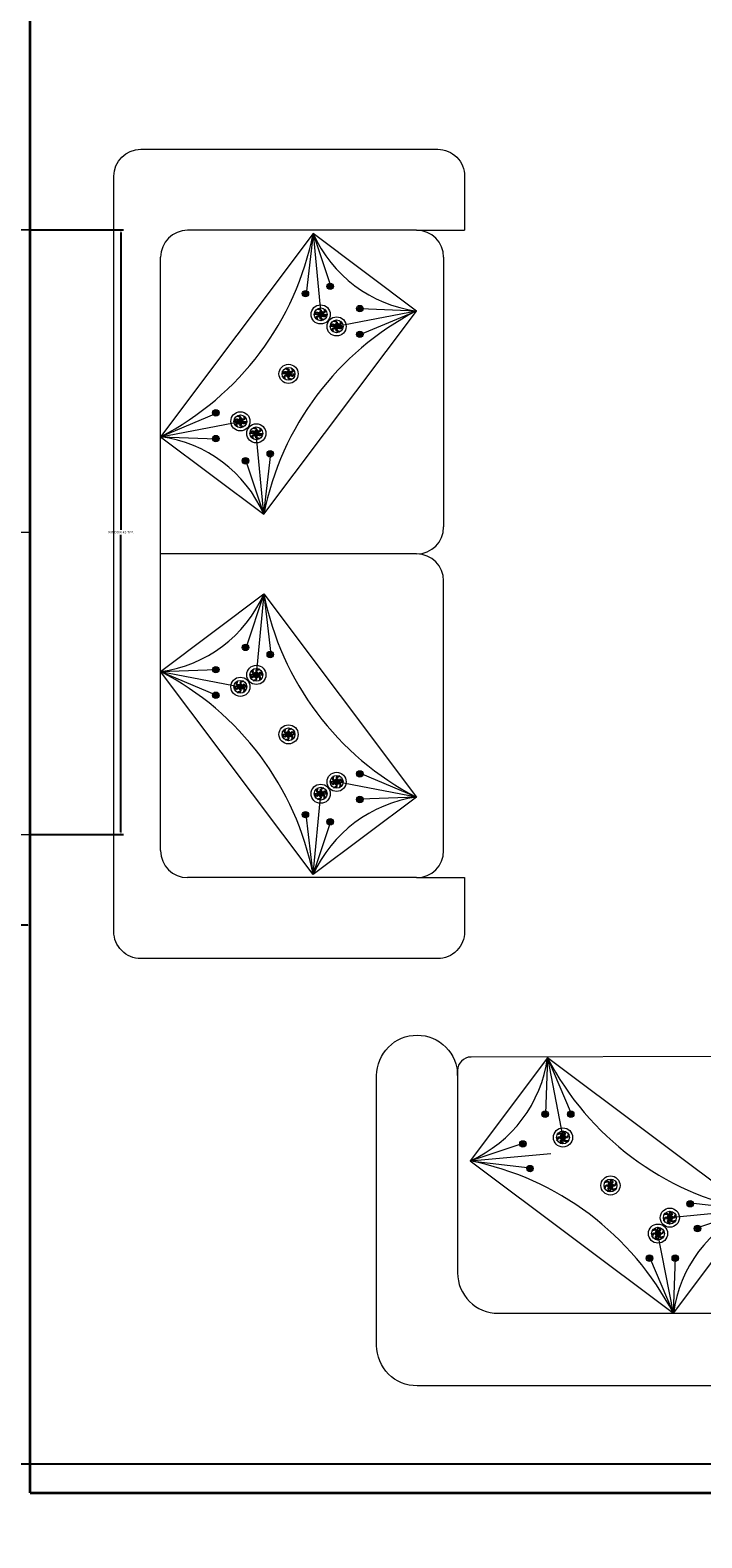
# Model space of a CAD drawing. Units: inches. Extents: x -61 to 1599, y -1316 to 257.
# Tile 193 of 204: x 1098 to 1147, y -173 to -61. Entities that reach past the tile are written whole.
import ezdxf

# ---------------------------------------------------------------- set-up
doc = ezdxf.new("R2010")
doc.units = ezdxf.units.IN
doc.header["$MEASUREMENT"] = 0
for name, color, linetype, lineweight in [('A-ANNO-DIMS', 2, 'Continuous', 18), ('FURNITURE', 83, 'Continuous', 18), ('WALLS', 4, 'Continuous', 35), ('WINDOWS', 220, 'Continuous', 18)]:
    doc.layers.add(name, color=color, linetype=linetype, lineweight=lineweight)
doc.layers.add('FUR', color=83, linetype='Continuous')
doc.styles.get("Standard").update_dxf_attribs({"font": 'arial.ttf'})
doc.dimstyles.get("Standard").update_dxf_attribs({"dimtxt": 0.18, "dimasz": 0.18, "dimexe": 0.18, "dimexo": 0.0625, "dimgap": 0.09, "dimtad": 0, "dimtih": 1, "dimtoh": 1, "dimdec": 0, "dimzin": 0, "dimdsep": 46, "dimlunit": 3, "dimtxsty": 'Standard', "dimcen": 0.09, "dimadec": 0, "dimazin": 0, "dimtfac": 1, "dimtdec": 0, "dimtofl": 0, "dimtmove": 0, "dimatfit": 3, "dimfxl": 1, "dimtolj": 1, "dimtzin": 0, "dimarcsym": 0})

# ---------------------------------------------------------------- blocks, each defined once
blk = doc.blocks.new('WIN-45IN')
for p, q in [((0, 44.83), (6, 44.83)), ((0, 0), (6, 0))]:
    blk.add_line(p, q)
for points in [[(6, 44.83), (3, 44.83), (3, 22.42), (6, 22.42)], [(3, 22.42), (0, 22.42), (0, 0), (3, 0)]]:
    blk.add_lwpolyline(points, close=True)
blk = doc.blocks.new('*U160')
at = {"layer": 'FUR'}
blk.add_open_spline([(0, 0.08), (-0.03, 0.05), (-0.1, -0.02), (0.08, -0.02), (0.02, -0.06), (0, -0.08)], degree=3, knots=[0, 0, 0, 0, 0.0954578, 0.1898773, 0.2470677, 0.2470677, 0.2470677, 0.2470677], dxfattribs=at)
blk = doc.blocks.new('*U161')
at = {"layer": 'FUR', "transparency": 16777216}
for p, rotation in [((222.17, -79.98), 60), ((222.18, -80.06), 120), ((222.31, -79.97), 300), ((222.25, -80.09), 180), ((222.32, -80.05), 240)]:
    blk.add_blockref('*U160', p, dxfattribs=dict(at, rotation=rotation))
blk.add_blockref('*U160', (222.24, -79.93), dxfattribs=at)
blk = doc.blocks.new('*U172')
at = {"layer": 'FUR'}
blk.add_open_spline([(0, 0.08), (-0.03, 0.05), (-0.1, -0.02), (0.08, -0.02), (0.02, -0.06), (0, -0.08)], degree=3, knots=[0, 0, 0, 0, 0.0954578, 0.1898773, 0.2470677, 0.2470677, 0.2470677, 0.2470677], dxfattribs=at)
blk = doc.blocks.new('*U173')
at = {"layer": 'FUR', "transparency": 16777216}
for p, rotation in [((222.17, -79.98), 60), ((222.18, -80.06), 120), ((222.31, -79.97), 300), ((222.25, -80.09), 180), ((222.32, -80.05), 240)]:
    blk.add_blockref('*U172', p, dxfattribs=dict(at, rotation=rotation))
blk.add_blockref('*U172', (222.24, -79.93), dxfattribs=at)
blk = doc.blocks.new('*U186')
at = {"layer": 'FUR'}
blk.add_open_spline([(0, 0.08), (-0.03, 0.05), (-0.1, -0.02), (0.08, -0.02), (0.02, -0.06), (0, -0.08)], degree=3, knots=[0, 0, 0, 0, 0.0954578, 0.1898773, 0.2470677, 0.2470677, 0.2470677, 0.2470677], dxfattribs=at)
blk = doc.blocks.new('*U187')
at = {"layer": 'FUR', "transparency": 16777216}
for p, rotation in [((222.17, -79.98), 60), ((222.18, -80.06), 120), ((222.31, -79.97), 300), ((222.25, -80.09), 180), ((222.32, -80.05), 240)]:
    blk.add_blockref('*U186', p, dxfattribs=dict(at, rotation=rotation))
blk.add_blockref('*U186', (222.24, -79.93), dxfattribs=at)
blk = doc.blocks.new('*U198')
at = {"layer": 'FUR'}
blk.add_open_spline([(0, 0.08), (-0.03, 0.05), (-0.1, -0.02), (0.08, -0.02), (0.02, -0.06), (0, -0.08)], degree=3, knots=[0, 0, 0, 0, 0.0954578, 0.1898773, 0.2470677, 0.2470677, 0.2470677, 0.2470677], dxfattribs=at)
blk = doc.blocks.new('*U199')
at = {"layer": 'FUR', "transparency": 16777216}
for p, rotation in [((222.17, -79.98), 60), ((222.18, -80.06), 120), ((222.31, -79.97), 300), ((222.25, -80.09), 180), ((222.32, -80.05), 240)]:
    blk.add_blockref('*U198', p, dxfattribs=dict(at, rotation=rotation))
blk.add_blockref('*U198', (222.24, -79.93), dxfattribs=at)
blk = doc.blocks.new('*U184')
at = {"layer": 'FUR'}
blk.add_open_spline([(0.01, 0.24), (-0.09, 0.14), (-0.29, -0.05), (0.22, -0.05), (0.07, -0.19), (0.01, -0.24)], degree=3, knots=[0, 0, 0, 0, 0.2846533, 0.5662105, 0.736751, 0.736751, 0.736751, 0.736751], dxfattribs=at)
blk = doc.blocks.new('*U159')
at = {"layer": 'FUR', "transparency": 16777216}
for p, rotation in [((662.52, -238.49), 60), ((662.53, -238.73), 120), ((662.74, -238.83), 180), ((662.93, -238.46), 300), ((662.94, -238.7), 240)]:
    blk.add_blockref('*U184', p, dxfattribs=dict(at, rotation=rotation))
blk.add_blockref('*U184', (662.72, -238.36), dxfattribs=at)
blk = doc.blocks.new('*U210')
at = {"layer": 'FUR'}
blk.add_open_spline([(0.01, 0.24), (-0.09, 0.14), (-0.29, -0.05), (0.22, -0.05), (0.07, -0.19), (0.01, -0.24)], degree=3, knots=[0, 0, 0, 0, 0.2846533, 0.5662105, 0.736751, 0.736751, 0.736751, 0.736751], dxfattribs=at)
blk = doc.blocks.new('*U185')
at = {"layer": 'FUR', "transparency": 16777216}
for p, rotation in [((662.52, -238.49), 60), ((662.53, -238.73), 120), ((662.74, -238.83), 180), ((662.93, -238.46), 300), ((662.94, -238.7), 240)]:
    blk.add_blockref('*U210', p, dxfattribs=dict(at, rotation=rotation))
blk.add_blockref('*U210', (662.72, -238.36), dxfattribs=at)
blk = doc.blocks.new('*U174')
at = {"layer": 'FUR'}
blk.add_open_spline([(0, 0.08), (-0.03, 0.05), (-0.1, -0.02), (0.08, -0.02), (0.02, -0.06), (0, -0.08)], degree=3, knots=[0, 0, 0, 0, 0.0954578, 0.1898773, 0.2470677, 0.2470677, 0.2470677, 0.2470677], dxfattribs=at)
blk = doc.blocks.new('*U175')
at = {"layer": 'FUR', "transparency": 16777216}
for p, rotation in [((222.17, -79.98), 60), ((222.18, -80.06), 120), ((222.31, -79.97), 300), ((222.25, -80.09), 180), ((222.32, -80.05), 240)]:
    blk.add_blockref('*U174', p, dxfattribs=dict(at, rotation=rotation))
blk.add_blockref('*U174', (222.24, -79.93), dxfattribs=at)
blk = doc.blocks.new('*U200')
at = {"layer": 'FUR'}
blk.add_open_spline([(0, 0.08), (-0.03, 0.05), (-0.1, -0.02), (0.08, -0.02), (0.02, -0.06), (0, -0.08)], degree=3, knots=[0, 0, 0, 0, 0.0954578, 0.1898773, 0.2470677, 0.2470677, 0.2470677, 0.2470677], dxfattribs=at)
blk = doc.blocks.new('*U201')
at = {"layer": 'FUR', "transparency": 16777216}
for p, rotation in [((222.17, -79.98), 60), ((222.18, -80.06), 120), ((222.31, -79.97), 300), ((222.25, -80.09), 180), ((222.32, -80.05), 240)]:
    blk.add_blockref('*U200', p, dxfattribs=dict(at, rotation=rotation))
blk.add_blockref('*U200', (222.24, -79.93), dxfattribs=at)
blk = doc.blocks.new('*U168')
at = {"layer": 'FUR'}
blk.add_open_spline([(0.01, 0.24), (-0.09, 0.14), (-0.29, -0.05), (0.22, -0.05), (0.07, -0.19), (0.01, -0.24)], degree=3, knots=[0, 0, 0, 0, 0.2846533, 0.5662105, 0.736751, 0.736751, 0.736751, 0.736751], dxfattribs=at)
blk = doc.blocks.new('*U169')
at = {"layer": 'FUR', "transparency": 16777216}
for p, rotation in [((662.52, -238.49), 60), ((662.53, -238.73), 120), ((662.74, -238.83), 180), ((662.93, -238.46), 300), ((662.94, -238.7), 240)]:
    blk.add_blockref('*U168', p, dxfattribs=dict(at, rotation=rotation))
blk.add_blockref('*U168', (662.72, -238.36), dxfattribs=at)
blk = doc.blocks.new('*U194')
at = {"layer": 'FUR'}
blk.add_open_spline([(0.01, 0.24), (-0.09, 0.14), (-0.29, -0.05), (0.22, -0.05), (0.07, -0.19), (0.01, -0.24)], degree=3, knots=[0, 0, 0, 0, 0.2846533, 0.5662105, 0.736751, 0.736751, 0.736751, 0.736751], dxfattribs=at)
blk = doc.blocks.new('*U195')
at = {"layer": 'FUR', "transparency": 16777216}
for p, rotation in [((662.52, -238.49), 60), ((662.53, -238.73), 120), ((662.74, -238.83), 180), ((662.93, -238.46), 300), ((662.94, -238.7), 240)]:
    blk.add_blockref('*U194', p, dxfattribs=dict(at, rotation=rotation))
blk.add_blockref('*U194', (662.72, -238.36), dxfattribs=at)
blk = doc.blocks.new('*U176')
at = {"layer": 'FUR'}
blk.add_open_spline([(0, 0.08), (-0.03, 0.05), (-0.1, -0.02), (0.08, -0.02), (0.02, -0.06), (0, -0.08)], degree=3, knots=[0, 0, 0, 0, 0.0954578, 0.1898773, 0.2470677, 0.2470677, 0.2470677, 0.2470677], dxfattribs=at)
blk = doc.blocks.new('*U177')
at = {"layer": 'FUR', "transparency": 16777216}
for p, rotation in [((222.17, -79.98), 60), ((222.18, -80.06), 120), ((222.31, -79.97), 300), ((222.25, -80.09), 180), ((222.32, -80.05), 240)]:
    blk.add_blockref('*U176', p, dxfattribs=dict(at, rotation=rotation))
blk.add_blockref('*U176', (222.24, -79.93), dxfattribs=at)
blk = doc.blocks.new('*U202')
at = {"layer": 'FUR'}
blk.add_open_spline([(0, 0.08), (-0.03, 0.05), (-0.1, -0.02), (0.08, -0.02), (0.02, -0.06), (0, -0.08)], degree=3, knots=[0, 0, 0, 0, 0.0954578, 0.1898773, 0.2470677, 0.2470677, 0.2470677, 0.2470677], dxfattribs=at)
blk = doc.blocks.new('*U203')
at = {"layer": 'FUR', "transparency": 16777216}
for p, rotation in [((222.17, -79.98), 60), ((222.18, -80.06), 120), ((222.31, -79.97), 300), ((222.25, -80.09), 180), ((222.32, -80.05), 240)]:
    blk.add_blockref('*U202', p, dxfattribs=dict(at, rotation=rotation))
blk.add_blockref('*U202', (222.24, -79.93), dxfattribs=at)
blk = doc.blocks.new('*U170')
at = {"layer": 'FUR'}
blk.add_open_spline([(0.01, 0.24), (-0.09, 0.14), (-0.29, -0.05), (0.22, -0.05), (0.07, -0.19), (0.01, -0.24)], degree=3, knots=[0, 0, 0, 0, 0.2846533, 0.5662105, 0.736751, 0.736751, 0.736751, 0.736751], dxfattribs=at)
blk = doc.blocks.new('*U171')
at = {"layer": 'FUR', "transparency": 16777216}
for p, rotation in [((662.52, -238.49), 60), ((662.53, -238.73), 120), ((662.74, -238.83), 180), ((662.93, -238.46), 300), ((662.94, -238.7), 240)]:
    blk.add_blockref('*U170', p, dxfattribs=dict(at, rotation=rotation))
blk.add_blockref('*U170', (662.72, -238.36), dxfattribs=at)
blk = doc.blocks.new('*U196')
at = {"layer": 'FUR'}
blk.add_open_spline([(0.01, 0.24), (-0.09, 0.14), (-0.29, -0.05), (0.22, -0.05), (0.07, -0.19), (0.01, -0.24)], degree=3, knots=[0, 0, 0, 0, 0.2846533, 0.5662105, 0.736751, 0.736751, 0.736751, 0.736751], dxfattribs=at)
blk = doc.blocks.new('*U197')
at = {"layer": 'FUR', "transparency": 16777216}
for p, rotation in [((662.52, -238.49), 60), ((662.53, -238.73), 120), ((662.74, -238.83), 180), ((662.93, -238.46), 300), ((662.94, -238.7), 240)]:
    blk.add_blockref('*U196', p, dxfattribs=dict(at, rotation=rotation))
blk.add_blockref('*U196', (662.72, -238.36), dxfattribs=at)
blk = doc.blocks.new('*U164')
at = {"layer": 'FUR'}
blk.add_open_spline([(0, 0.08), (-0.03, 0.05), (-0.1, -0.02), (0.08, -0.02), (0.02, -0.06), (0, -0.08)], degree=3, knots=[0, 0, 0, 0, 0.0954578, 0.1898773, 0.2470677, 0.2470677, 0.2470677, 0.2470677], dxfattribs=at)
blk = doc.blocks.new('*U165')
at = {"layer": 'FUR', "transparency": 16777216}
for p, rotation in [((222.17, -79.98), 60), ((222.18, -80.06), 120), ((222.31, -79.97), 300), ((222.25, -80.09), 180), ((222.32, -80.05), 240)]:
    blk.add_blockref('*U164', p, dxfattribs=dict(at, rotation=rotation))
blk.add_blockref('*U164', (222.24, -79.93), dxfattribs=at)
blk = doc.blocks.new('*U190')
at = {"layer": 'FUR'}
blk.add_open_spline([(0, 0.08), (-0.03, 0.05), (-0.1, -0.02), (0.08, -0.02), (0.02, -0.06), (0, -0.08)], degree=3, knots=[0, 0, 0, 0, 0.0954578, 0.1898773, 0.2470677, 0.2470677, 0.2470677, 0.2470677], dxfattribs=at)
blk = doc.blocks.new('*U191')
at = {"layer": 'FUR', "transparency": 16777216}
for p, rotation in [((222.17, -79.98), 60), ((222.18, -80.06), 120), ((222.31, -79.97), 300), ((222.25, -80.09), 180), ((222.32, -80.05), 240)]:
    blk.add_blockref('*U190', p, dxfattribs=dict(at, rotation=rotation))
blk.add_blockref('*U190', (222.24, -79.93), dxfattribs=at)
blk = doc.blocks.new('*U183')
at = {"layer": 'FUR'}
blk.add_open_spline([(0.01, 0.24), (-0.09, 0.14), (-0.29, -0.05), (0.22, -0.05), (0.07, -0.19), (0.01, -0.24)], degree=3, knots=[0, 0, 0, 0, 0.2846533, 0.5662105, 0.736751, 0.736751, 0.736751, 0.736751], dxfattribs=at)
blk = doc.blocks.new('*U162')
at = {"layer": 'FUR', "transparency": 16777216}
for p, rotation in [((662.52, -238.49), 60), ((662.53, -238.73), 120), ((662.74, -238.83), 180), ((662.93, -238.46), 300), ((662.94, -238.7), 240)]:
    blk.add_blockref('*U183', p, dxfattribs=dict(at, rotation=rotation))
blk.add_blockref('*U183', (662.72, -238.36), dxfattribs=at)
blk = doc.blocks.new('*U209')
at = {"layer": 'FUR'}
blk.add_open_spline([(0.01, 0.24), (-0.09, 0.14), (-0.29, -0.05), (0.22, -0.05), (0.07, -0.19), (0.01, -0.24)], degree=3, knots=[0, 0, 0, 0, 0.2846533, 0.5662105, 0.736751, 0.736751, 0.736751, 0.736751], dxfattribs=at)
blk = doc.blocks.new('*U188')
at = {"layer": 'FUR', "transparency": 16777216}
for p, rotation in [((662.52, -238.49), 60), ((662.53, -238.73), 120), ((662.74, -238.83), 180), ((662.93, -238.46), 300), ((662.94, -238.7), 240)]:
    blk.add_blockref('*U209', p, dxfattribs=dict(at, rotation=rotation))
blk.add_blockref('*U209', (662.72, -238.36), dxfattribs=at)
blk = doc.blocks.new('*U182')
at = {"layer": 'FUR'}
blk.add_open_spline([(0, 0.08), (-0.03, 0.05), (-0.1, -0.02), (0.08, -0.02), (0.02, -0.06), (0, -0.08)], degree=3, knots=[0, 0, 0, 0, 0.0954578, 0.1898773, 0.2470677, 0.2470677, 0.2470677, 0.2470677], dxfattribs=at)
blk = doc.blocks.new('*U163')
at = {"layer": 'FUR', "transparency": 16777216}
for p, rotation in [((222.17, -79.98), 60), ((222.18, -80.06), 120), ((222.31, -79.97), 300), ((222.25, -80.09), 180), ((222.32, -80.05), 240)]:
    blk.add_blockref('*U182', p, dxfattribs=dict(at, rotation=rotation))
blk.add_blockref('*U182', (222.24, -79.93), dxfattribs=at)
blk = doc.blocks.new('*U208')
at = {"layer": 'FUR'}
blk.add_open_spline([(0, 0.08), (-0.03, 0.05), (-0.1, -0.02), (0.08, -0.02), (0.02, -0.06), (0, -0.08)], degree=3, knots=[0, 0, 0, 0, 0.0954578, 0.1898773, 0.2470677, 0.2470677, 0.2470677, 0.2470677], dxfattribs=at)
blk = doc.blocks.new('*U189')
at = {"layer": 'FUR', "transparency": 16777216}
for p, rotation in [((222.17, -79.98), 60), ((222.18, -80.06), 120), ((222.31, -79.97), 300), ((222.25, -80.09), 180), ((222.32, -80.05), 240)]:
    blk.add_blockref('*U208', p, dxfattribs=dict(at, rotation=rotation))
blk.add_blockref('*U208', (222.24, -79.93), dxfattribs=at)
blk = doc.blocks.new('*U166')
at = {"layer": 'FUR'}
blk.add_open_spline([(0.01, 0.24), (-0.09, 0.14), (-0.29, -0.05), (0.22, -0.05), (0.07, -0.19), (0.01, -0.24)], degree=3, knots=[0, 0, 0, 0, 0.2846533, 0.5662105, 0.736751, 0.736751, 0.736751, 0.736751], dxfattribs=at)
blk = doc.blocks.new('*U167')
at = {"layer": 'FUR', "transparency": 16777216}
for p, rotation in [((662.52, -238.49), 60), ((662.53, -238.73), 120), ((662.74, -238.83), 180), ((662.93, -238.46), 300), ((662.94, -238.7), 240)]:
    blk.add_blockref('*U166', p, dxfattribs=dict(at, rotation=rotation))
blk.add_blockref('*U166', (662.72, -238.36), dxfattribs=at)
blk = doc.blocks.new('*U192')
at = {"layer": 'FUR'}
blk.add_open_spline([(0.01, 0.24), (-0.09, 0.14), (-0.29, -0.05), (0.22, -0.05), (0.07, -0.19), (0.01, -0.24)], degree=3, knots=[0, 0, 0, 0, 0.2846533, 0.5662105, 0.736751, 0.736751, 0.736751, 0.736751], dxfattribs=at)
blk = doc.blocks.new('*U193')
at = {"layer": 'FUR', "transparency": 16777216}
for p, rotation in [((662.52, -238.49), 60), ((662.53, -238.73), 120), ((662.74, -238.83), 180), ((662.93, -238.46), 300), ((662.94, -238.7), 240)]:
    blk.add_blockref('*U192', p, dxfattribs=dict(at, rotation=rotation))
blk.add_blockref('*U192', (662.72, -238.36), dxfattribs=at)
blk = doc.blocks.new('*U178')
at = {"layer": 'FUR'}
blk.add_open_spline([(0, 0.08), (-0.03, 0.05), (-0.1, -0.02), (0.08, -0.02), (0.02, -0.06), (0, -0.08)], degree=3, knots=[0, 0, 0, 0, 0.0954578, 0.1898773, 0.2470677, 0.2470677, 0.2470677, 0.2470677], dxfattribs=at)
blk = doc.blocks.new('*U179')
at = {"layer": 'FUR', "transparency": 16777216}
for p, rotation in [((222.17, -79.98), 60), ((222.18, -80.06), 120), ((222.31, -79.97), 300), ((222.25, -80.09), 180), ((222.32, -80.05), 240)]:
    blk.add_blockref('*U178', p, dxfattribs=dict(at, rotation=rotation))
blk.add_blockref('*U178', (222.24, -79.93), dxfattribs=at)
blk = doc.blocks.new('*U180')
at = {"layer": 'FUR'}
blk.add_open_spline([(0, 0.08), (-0.03, 0.05), (-0.1, -0.02), (0.08, -0.02), (0.02, -0.06), (0, -0.08)], degree=3, knots=[0, 0, 0, 0, 0.0954578, 0.1898773, 0.2470677, 0.2470677, 0.2470677, 0.2470677], dxfattribs=at)
blk = doc.blocks.new('*U181')
at = {"layer": 'FUR', "transparency": 16777216}
for p, rotation in [((222.17, -79.98), 60), ((222.18, -80.06), 120), ((222.31, -79.97), 300), ((222.25, -80.09), 180), ((222.32, -80.05), 240)]:
    blk.add_blockref('*U180', p, dxfattribs=dict(at, rotation=rotation))
blk.add_blockref('*U180', (222.24, -79.93), dxfattribs=at)
blk = doc.blocks.new('*U204')
at = {"layer": 'FUR'}
blk.add_open_spline([(0, 0.08), (-0.03, 0.05), (-0.1, -0.02), (0.08, -0.02), (0.02, -0.06), (0, -0.08)], degree=3, knots=[0, 0, 0, 0, 0.0954578, 0.1898773, 0.2470677, 0.2470677, 0.2470677, 0.2470677], dxfattribs=at)
blk = doc.blocks.new('*U205')
at = {"layer": 'FUR', "transparency": 16777216}
for p, rotation in [((222.17, -79.98), 60), ((222.18, -80.06), 120), ((222.31, -79.97), 300), ((222.25, -80.09), 180), ((222.32, -80.05), 240)]:
    blk.add_blockref('*U204', p, dxfattribs=dict(at, rotation=rotation))
blk.add_blockref('*U204', (222.24, -79.93), dxfattribs=at)
blk = doc.blocks.new('*U206')
at = {"layer": 'FUR'}
blk.add_open_spline([(0, 0.08), (-0.03, 0.05), (-0.1, -0.02), (0.08, -0.02), (0.02, -0.06), (0, -0.08)], degree=3, knots=[0, 0, 0, 0, 0.0954578, 0.1898773, 0.2470677, 0.2470677, 0.2470677, 0.2470677], dxfattribs=at)
blk = doc.blocks.new('*U207')
at = {"layer": 'FUR', "transparency": 16777216}
for p, rotation in [((222.17, -79.98), 60), ((222.18, -80.06), 120), ((222.31, -79.97), 300), ((222.25, -80.09), 180), ((222.32, -80.05), 240)]:
    blk.add_blockref('*U206', p, dxfattribs=dict(at, rotation=rotation))
blk.add_blockref('*U206', (222.24, -79.93), dxfattribs=at)
blk = doc.blocks.new('SOFA-LOVESEAT')
for p, q in [((22.44, 54), (5.47, 54)), ((14.78, 53.75), (14.25, 49.29)), ((14.78, 53.75), (15.33, 47.76)), ((14.78, 53.75), (16.08, 49.82)), ((22.44, 54), (26, 54)), ((3.47, 8), (3.47, 52)), ((24.44, 52), (24.44, 32)), ((14.2, 49.3), (14.04, 49.3)), ((14.2, 49.3), (14.36, 49.3)), ((16.03, 49.84), (15.87, 49.84)), ((16.03, 49.84), (16.19, 49.84)), ((18.23, 48.19), (18.07, 48.19)), ((18.23, 48.19), (18.39, 48.19)), ((22.42, 48.01), (18.28, 48.17)), ((15.33, 47.76), (14.86, 47.76)), ((15.33, 47.76), (15.81, 47.76)), ((22.42, 48.01), (16.51, 46.87)), ((22.42, 48.01), (18.28, 46.26)), ((16.51, 46.87), (16.03, 46.87)), ((16.51, 46.87), (16.99, 46.87)), ((18.23, 46.28), (18.07, 46.28)), ((18.23, 46.28), (18.39, 46.28)), ((12.95, 43.35), (12.47, 43.35)), ((12.95, 43.35), (13.42, 43.35)), ((3.47, 38.69), (7.61, 40.44)), ((7.56, 40.46), (7.4, 40.46)), ((7.56, 40.46), (7.72, 40.46)), ((3.47, 38.69), (9.38, 39.83)), ((9.38, 39.83), (8.9, 39.83)), ((9.38, 39.83), (9.86, 39.83)), ((3.47, 38.69), (7.61, 38.53)), ((7.56, 38.55), (7.4, 38.55)), ((7.56, 38.55), (7.72, 38.55)), ((10.56, 38.94), (10.08, 38.94)), ((11.12, 32.95), (10.56, 38.94)), ((10.56, 38.94), (11.04, 38.94)), ((9.76, 36.9), (9.6, 36.9)), ((9.76, 36.9), (9.92, 36.9)), ((11.12, 32.95), (11.64, 37.41)), ((11.59, 37.43), (11.43, 37.43)), ((11.59, 37.43), (11.75, 37.43)), ((11.12, 32.95), (9.81, 36.88)), ((22.44, 30), (3.47, 30)), ((22.44, 30), (22.44, 30)), ((24.44, 8), (24.44, 28)), ((11.12, 27.03), (9.81, 23.09)), ((11.12, 27.03), (10.56, 21.03)), ((11.12, 27.03), (11.64, 22.56)), ((9.76, 23.07), (9.6, 23.07)), ((9.76, 23.07), (9.92, 23.07)), ((11.59, 22.54), (11.43, 22.54)), ((11.59, 22.54), (11.75, 22.54)), ((3.47, 21.29), (7.61, 21.44)), ((3.47, 21.29), (9.38, 20.15)), ((3.47, 21.29), (7.61, 19.54)), ((7.56, 21.42), (7.4, 21.42)), ((7.56, 21.42), (7.72, 21.42)), ((9.38, 20.15), (8.9, 20.15)), ((9.38, 20.15), (9.86, 20.15)), ((10.56, 21.03), (10.08, 21.03)), ((10.56, 21.03), (11.04, 21.03)), ((7.56, 19.52), (7.4, 19.52)), ((7.56, 19.52), (7.72, 19.52)), ((12.95, 16.62), (12.47, 16.62)), ((12.95, 16.62), (13.42, 16.62)), ((18.23, 13.69), (18.07, 13.69)), ((18.23, 13.69), (18.39, 13.69)), ((22.42, 11.96), (18.28, 13.71)), ((16.51, 13.1), (16.03, 13.1)), ((22.42, 11.96), (16.51, 13.1)), ((16.51, 13.1), (16.99, 13.1)), ((14.78, 6.22), (15.33, 12.22)), ((15.33, 12.22), (14.86, 12.22)), ((15.33, 12.22), (15.81, 12.22)), ((18.23, 11.79), (18.07, 11.79)), ((18.23, 11.79), (18.39, 11.79)), ((22.42, 11.96), (18.28, 11.81)), ((14.2, 10.67), (14.04, 10.67)), ((14.2, 10.67), (14.36, 10.67)), ((14.78, 6.22), (14.25, 10.69)), ((14.78, 6.22), (16.08, 10.16)), ((16.03, 10.14), (15.87, 10.14)), ((16.03, 10.14), (16.19, 10.14)), ((22.44, 6), (5.47, 6)), ((22.44, 6), (26, 6))]:
    blk.add_line(p, q)
blk.add_lwpolyline([(26, 6), (26, 2, -0.414214), (24, 0), (2, 0, -0.414214), (0, 2), (0, 58, -0.414213), (2, 60), (24, 60, -0.414214), (26, 58), (26, 54)], format="xyb")
for points in [[(11.12, 32.95), (22.42, 48.01), (14.78, 53.75), (3.47, 38.69)], [(11.12, 27.03), (22.42, 11.96), (14.78, 6.22), (3.47, 21.29)]]:
    blk.add_lwpolyline(points, close=True)
for centre, radius in [((14.2, 49.3), 0.238), ((14.2, 49.3), 0.16), ((16.03, 49.84), 0.238), ((16.03, 49.84), 0.16), ((15.33, 47.76), 0.71), ((15.33, 47.76), 0.476), ((18.23, 48.19), 0.238), ((18.23, 48.19), 0.16), ((16.51, 46.87), 0.71), ((16.51, 46.87), 0.476), ((18.23, 46.28), 0.238), ((18.23, 46.28), 0.16), ((12.95, 43.35), 0.71), ((12.95, 43.35), 0.476), ((7.56, 40.46), 0.238), ((7.56, 40.46), 0.16), ((9.38, 39.83), 0.71), ((9.38, 39.83), 0.476), ((10.56, 38.94), 0.71), ((10.56, 38.94), 0.476), ((7.56, 38.55), 0.238), ((7.56, 38.55), 0.16), ((9.76, 36.9), 0.238), ((9.76, 36.9), 0.16), ((11.59, 37.43), 0.238), ((11.59, 37.43), 0.16), ((9.76, 23.07), 0.238), ((9.76, 23.07), 0.16), ((11.59, 22.54), 0.238), ((11.59, 22.54), 0.16), ((7.56, 21.42), 0.238), ((7.56, 21.42), 0.16), ((10.56, 21.03), 0.71), ((10.56, 21.03), 0.476), ((9.38, 20.15), 0.71), ((9.38, 20.15), 0.476), ((7.56, 19.52), 0.238), ((7.56, 19.52), 0.16), ((12.95, 16.62), 0.71), ((12.95, 16.62), 0.476), ((16.51, 13.1), 0.71), ((16.51, 13.1), 0.476), ((18.23, 13.69), 0.238), ((18.23, 13.69), 0.16), ((15.33, 12.22), 0.71), ((15.33, 12.22), 0.476), ((18.23, 11.79), 0.238), ((18.23, 11.79), 0.16), ((14.2, 10.67), 0.238), ((14.2, 10.67), 0.16), ((16.03, 10.14), 0.238), ((16.03, 10.14), 0.16)]:
    blk.add_circle(centre, radius)
for centre, radius, start, end in [((5.47, 52), 2, 90, 180), ((-6.54, 57.97), 21.73, 297.4317, 348.7956), ((23.75, 57.74), 9.82, 203.9742, 262.253), ((22.44, 52), 2, 0, 90), ((32.43, 28.73), 21.73, 117.4317, 168.7956), ((2.15, 28.96), 9.82, 23.9742, 82.253), ((22.44, 32), 2, 270, 0), ((22.44, 28), 2, 0, 90), ((2.15, 31.01), 9.82, 277.747, 336.0258), ((32.43, 31.25), 21.73, 191.2044, 242.5684), ((-6.54, 2), 21.73, 11.2044, 62.5684), ((23.75, 2.23), 9.82, 97.747, 156.0258), ((5.47, 8), 2, 180, 270), ((22.44, 8), 2, 270, 0)]:
    blk.add_arc(centre, radius, start, end)
at = {"xscale": -1, "rotation": 90.00003000000098}
for name, p in [('*U191', (-65.81, 271.55)), ('*U189', (-63.98, 272.08)), ('*U188', (-223.26, 710.49)), ('*U205', (-61.78, 270.43)), ('*U193', (-222.08, 709.6)), ('*U207', (-61.78, 268.53)), ('*U197', (-225.65, 706.08)), ('*U187', (-72.45, 262.7)), ('*U185', (-229.21, 702.56)), ('*U195', (-228.03, 701.67)), ('*U199', (-72.45, 260.8)), ('*U201', (-70.25, 259.15)), ('*U203', (-68.43, 259.68))]:
    blk.add_blockref(name, p, dxfattribs=at)
at = {"rotation": 90}
for name, p in [('*U175', (-70.25, -199.17)), ('*U177', (-68.43, -199.7)), ('*U173', (-72.45, -200.82)), ('*U169', (-228.03, -641.7)), ('*U159', (-229.21, -642.58)), ('*U161', (-72.45, -202.73)), ('*U171', (-225.65, -646.11)), ('*U167', (-222.08, -649.63)), ('*U181', (-61.78, -208.55)), ('*U162', (-223.26, -650.51)), ('*U179', (-61.78, -210.46)), ('*U165', (-65.81, -211.58)), ('*U163', (-63.98, -212.11))]:
    blk.add_blockref(name, p, dxfattribs=at)
blk = doc.blocks.new('*U152')
at = {"layer": 'FUR'}
blk.add_open_spline([(0, 0.08), (-0.03, 0.05), (-0.1, -0.02), (0.08, -0.02), (0.02, -0.06), (0, -0.08)], degree=3, knots=[0, 0, 0, 0, 0.0954578, 0.1898773, 0.2470677, 0.2470677, 0.2470677, 0.2470677], dxfattribs=at)
blk = doc.blocks.new('*U153')
at = {"layer": 'FUR', "transparency": 16777216}
for p, rotation in [((222.17, -79.98), 60), ((222.18, -80.06), 120), ((222.31, -79.97), 300), ((222.25, -80.09), 180), ((222.32, -80.05), 240)]:
    blk.add_blockref('*U152', p, dxfattribs=dict(at, rotation=rotation))
blk.add_blockref('*U152', (222.24, -79.93), dxfattribs=at)
blk = doc.blocks.new('*U154')
at = {"layer": 'FUR'}
blk.add_open_spline([(0, 0.08), (-0.03, 0.05), (-0.1, -0.02), (0.08, -0.02), (0.02, -0.06), (0, -0.08)], degree=3, knots=[0, 0, 0, 0, 0.0954578, 0.1898773, 0.2470677, 0.2470677, 0.2470677, 0.2470677], dxfattribs=at)
blk = doc.blocks.new('*U155')
at = {"layer": 'FUR', "transparency": 16777216}
for p, rotation in [((222.17, -79.98), 60), ((222.18, -80.06), 120), ((222.31, -79.97), 300), ((222.25, -80.09), 180), ((222.32, -80.05), 240)]:
    blk.add_blockref('*U154', p, dxfattribs=dict(at, rotation=rotation))
blk.add_blockref('*U154', (222.24, -79.93), dxfattribs=at)
blk = doc.blocks.new('*U148')
at = {"layer": 'FUR'}
blk.add_open_spline([(0, 0.08), (-0.03, 0.05), (-0.1, -0.02), (0.08, -0.02), (0.02, -0.06), (0, -0.08)], degree=3, knots=[0, 0, 0, 0, 0.0954578, 0.1898773, 0.2470677, 0.2470677, 0.2470677, 0.2470677], dxfattribs=at)
blk = doc.blocks.new('*U149')
at = {"layer": 'FUR', "transparency": 16777216}
for p, rotation in [((222.17, -79.98), 60), ((222.18, -80.06), 120), ((222.31, -79.97), 300), ((222.25, -80.09), 180), ((222.32, -80.05), 240)]:
    blk.add_blockref('*U148', p, dxfattribs=dict(at, rotation=rotation))
blk.add_blockref('*U148', (222.24, -79.93), dxfattribs=at)
blk = doc.blocks.new('*U128')
at = {"layer": 'FUR'}
blk.add_open_spline([(0.01, 0.24), (-0.09, 0.14), (-0.29, -0.05), (0.22, -0.05), (0.07, -0.19), (0.01, -0.24)], degree=3, knots=[0, 0, 0, 0, 0.2846533, 0.5662105, 0.736751, 0.736751, 0.736751, 0.736751], dxfattribs=at)
blk = doc.blocks.new('*U129')
at = {"layer": 'FUR', "transparency": 16777216}
for p, rotation in [((662.52, -238.49), 60), ((662.53, -238.73), 120), ((662.74, -238.83), 180), ((662.93, -238.46), 300), ((662.94, -238.7), 240)]:
    blk.add_blockref('*U128', p, dxfattribs=dict(at, rotation=rotation))
blk.add_blockref('*U128', (662.72, -238.36), dxfattribs=at)
blk = doc.blocks.new('*U150')
at = {"layer": 'FUR'}
blk.add_open_spline([(0, 0.08), (-0.03, 0.05), (-0.1, -0.02), (0.08, -0.02), (0.02, -0.06), (0, -0.08)], degree=3, knots=[0, 0, 0, 0, 0.0954578, 0.1898773, 0.2470677, 0.2470677, 0.2470677, 0.2470677], dxfattribs=at)
blk = doc.blocks.new('*U151')
at = {"layer": 'FUR', "transparency": 16777216}
for p, rotation in [((222.17, -79.98), 60), ((222.18, -80.06), 120), ((222.31, -79.97), 300), ((222.25, -80.09), 180), ((222.32, -80.05), 240)]:
    blk.add_blockref('*U150', p, dxfattribs=dict(at, rotation=rotation))
blk.add_blockref('*U150', (222.24, -79.93), dxfattribs=at)
blk = doc.blocks.new('*U132')
at = {"layer": 'FUR'}
blk.add_open_spline([(0.01, 0.24), (-0.09, 0.14), (-0.29, -0.05), (0.22, -0.05), (0.07, -0.19), (0.01, -0.24)], degree=3, knots=[0, 0, 0, 0, 0.2846533, 0.5662105, 0.736751, 0.736751, 0.736751, 0.736751], dxfattribs=at)
blk = doc.blocks.new('*U133')
at = {"layer": 'FUR', "transparency": 16777216}
for p, rotation in [((662.52, -238.49), 60), ((662.53, -238.73), 120), ((662.74, -238.83), 180), ((662.93, -238.46), 300), ((662.94, -238.7), 240)]:
    blk.add_blockref('*U132', p, dxfattribs=dict(at, rotation=rotation))
blk.add_blockref('*U132', (662.72, -238.36), dxfattribs=at)
blk = doc.blocks.new('*U124')
at = {"layer": 'FUR'}
blk.add_open_spline([(0, 0.08), (-0.03, 0.05), (-0.1, -0.02), (0.08, -0.02), (0.02, -0.06), (0, -0.08)], degree=3, knots=[0, 0, 0, 0, 0.0954578, 0.1898773, 0.2470677, 0.2470677, 0.2470677, 0.2470677], dxfattribs=at)
blk = doc.blocks.new('*U125')
at = {"layer": 'FUR', "transparency": 16777216}
for p, rotation in [((222.17, -79.98), 60), ((222.18, -80.06), 120), ((222.31, -79.97), 300), ((222.25, -80.09), 180), ((222.32, -80.05), 240)]:
    blk.add_blockref('*U124', p, dxfattribs=dict(at, rotation=rotation))
blk.add_blockref('*U124', (222.24, -79.93), dxfattribs=at)
blk = doc.blocks.new('*U134')
at = {"layer": 'FUR'}
blk.add_open_spline([(0.01, 0.24), (-0.09, 0.14), (-0.29, -0.05), (0.22, -0.05), (0.07, -0.19), (0.01, -0.24)], degree=3, knots=[0, 0, 0, 0, 0.2846533, 0.5662105, 0.736751, 0.736751, 0.736751, 0.736751], dxfattribs=at)
blk = doc.blocks.new('*U123')
at = {"layer": 'FUR', "transparency": 16777216}
for p, rotation in [((662.52, -238.49), 60), ((662.53, -238.73), 120), ((662.74, -238.83), 180), ((662.93, -238.46), 300), ((662.94, -238.7), 240)]:
    blk.add_blockref('*U134', p, dxfattribs=dict(at, rotation=rotation))
blk.add_blockref('*U134', (662.72, -238.36), dxfattribs=at)
blk = doc.blocks.new('*U130')
at = {"layer": 'FUR'}
blk.add_open_spline([(0.01, 0.24), (-0.09, 0.14), (-0.29, -0.05), (0.22, -0.05), (0.07, -0.19), (0.01, -0.24)], degree=3, knots=[0, 0, 0, 0, 0.2846533, 0.5662105, 0.736751, 0.736751, 0.736751, 0.736751], dxfattribs=at)
blk = doc.blocks.new('*U131')
at = {"layer": 'FUR', "transparency": 16777216}
for p, rotation in [((662.52, -238.49), 60), ((662.53, -238.73), 120), ((662.74, -238.83), 180), ((662.93, -238.46), 300), ((662.94, -238.7), 240)]:
    blk.add_blockref('*U130', p, dxfattribs=dict(at, rotation=rotation))
blk.add_blockref('*U130', (662.72, -238.36), dxfattribs=at)
blk = doc.blocks.new('*U126')
at = {"layer": 'FUR'}
blk.add_open_spline([(0, 0.08), (-0.03, 0.05), (-0.1, -0.02), (0.08, -0.02), (0.02, -0.06), (0, -0.08)], degree=3, knots=[0, 0, 0, 0, 0.0954578, 0.1898773, 0.2470677, 0.2470677, 0.2470677, 0.2470677], dxfattribs=at)
blk = doc.blocks.new('*U127')
at = {"layer": 'FUR', "transparency": 16777216}
for p, rotation in [((222.17, -79.98), 60), ((222.18, -80.06), 120), ((222.31, -79.97), 300), ((222.25, -80.09), 180), ((222.32, -80.05), 240)]:
    blk.add_blockref('*U126', p, dxfattribs=dict(at, rotation=rotation))
blk.add_blockref('*U126', (222.24, -79.93), dxfattribs=at)
blk = doc.blocks.new('*U146')
at = {"layer": 'FUR'}
blk.add_open_spline([(0, 0.08), (-0.03, 0.05), (-0.1, -0.02), (0.08, -0.02), (0.02, -0.06), (0, -0.08)], degree=3, knots=[0, 0, 0, 0, 0.0954578, 0.1898773, 0.2470677, 0.2470677, 0.2470677, 0.2470677], dxfattribs=at)
blk = doc.blocks.new('*U147')
at = {"layer": 'FUR', "transparency": 16777216}
for p, rotation in [((222.17, -79.98), 60), ((222.18, -80.06), 120), ((222.31, -79.97), 300), ((222.25, -80.09), 180), ((222.32, -80.05), 240)]:
    blk.add_blockref('*U146', p, dxfattribs=dict(at, rotation=rotation))
blk.add_blockref('*U146', (222.24, -79.93), dxfattribs=at)
blk = doc.blocks.new('*U144')
at = {"layer": 'FUR'}
blk.add_open_spline([(0, 0.08), (-0.03, 0.05), (-0.1, -0.02), (0.08, -0.02), (0.02, -0.06), (0, -0.08)], degree=3, knots=[0, 0, 0, 0, 0.0954578, 0.1898773, 0.2470677, 0.2470677, 0.2470677, 0.2470677], dxfattribs=at)
blk = doc.blocks.new('*U145')
at = {"layer": 'FUR', "transparency": 16777216}
for p, rotation in [((222.17, -79.98), 60), ((222.18, -80.06), 120), ((222.31, -79.97), 300), ((222.25, -80.09), 180), ((222.32, -80.05), 240)]:
    blk.add_blockref('*U144', p, dxfattribs=dict(at, rotation=rotation))
blk.add_blockref('*U144', (222.24, -79.93), dxfattribs=at)
blk = doc.blocks.new('SOFA-THREE-SEAT')
for p, q in [((30, 24.44), (7, 24.38)), ((12.66, 24.33), (12.51, 20.19)), ((12.66, 24.33), (13.81, 18.42)), ((12.66, 24.33), (14.41, 20.19)), ((6, 23), (6, 23.38)), ((12.49, 20.14), (12.49, 20.3)), ((12.49, 20.14), (12.49, 19.98)), ((14.39, 20.14), (14.39, 20.3)), ((14.39, 20.14), (14.39, 19.98)), ((6.93, 16.69), (10.86, 17.99)), ((10.84, 17.94), (10.84, 18.1)), ((10.84, 17.94), (10.84, 17.78)), ((13.81, 18.42), (13.81, 18.9)), ((13.81, 18.42), (13.81, 17.95)), ((6.93, 16.69), (12.92, 17.24)), ((6.93, 16.69), (11.39, 16.16)), ((11.37, 16.11), (11.37, 16.27)), ((11.37, 16.11), (11.37, 15.95)), ((17.33, 14.86), (17.33, 15.33)), ((17.33, 14.86), (17.33, 14.38)), ((23.24, 13.5), (23.24, 13.66)), ((23.24, 13.5), (23.24, 13.34)), ((27.73, 13.03), (23.26, 13.55)), ((27.73, 13.03), (21.73, 12.47)), ((21.73, 12.47), (21.73, 12.95)), ((21.73, 12.47), (21.73, 12)), ((27.73, 13.03), (23.79, 11.72)), ((20.85, 11.29), (20.85, 11.77)), ((21.99, 5.38), (20.85, 11.29)), ((20.85, 11.29), (20.85, 10.82)), ((23.78, 11.67), (23.78, 11.83)), ((23.78, 11.67), (23.78, 11.51)), ((20.22, 9.47), (20.22, 9.63)), ((20.22, 9.47), (20.22, 9.31)), ((21.99, 5.38), (20.24, 9.52)), ((21.99, 5.38), (22.14, 9.52)), ((22.13, 9.47), (22.13, 9.63)), ((22.13, 9.47), (22.13, 9.31))]:
    blk.add_line(p, q)
blk.add_lwpolyline([(78, 8.38), (78, 23, -0.414214), (81, 26), (81, 26, -0.414214), (84, 23), (84, 3, -0.414214), (81, 0), (3, 0, -0.414214), (0, 3), (0, 23, -0.414214), (3, 26), (3, 26, -0.414214), (6, 23), (6, 8.38, 0.414214), (9, 5.38), (75, 5.38, 0.414214)], format="xyb", close=True)
blk.add_lwpolyline([(27.73, 13.03), (12.66, 24.33), (6.93, 16.69), (21.99, 5.38)], close=True)
for centre, radius in [((12.49, 20.14), 0.238), ((12.49, 20.14), 0.16), ((14.39, 20.14), 0.238), ((14.39, 20.14), 0.16), ((13.81, 18.42), 0.71), ((10.84, 17.94), 0.238), ((10.84, 17.94), 0.16), ((13.81, 18.42), 0.476), ((11.37, 16.11), 0.238), ((11.37, 16.11), 0.16), ((17.33, 14.86), 0.71), ((17.33, 14.86), 0.476), ((23.24, 13.5), 0.238), ((23.24, 13.5), 0.16), ((21.73, 12.47), 0.71), ((21.73, 12.47), 0.476), ((20.85, 11.29), 0.71), ((20.85, 11.29), 0.476), ((23.78, 11.67), 0.238), ((23.78, 11.67), 0.16), ((20.22, 9.47), 0.238), ((20.22, 9.47), 0.16), ((22.13, 9.47), 0.238), ((22.13, 9.47), 0.16)]:
    blk.add_circle(centre, radius)
for centre, radius, start, end in [((7, 23.38), 1, 90.1542, 180.1542), ((2.94, 25.66), 9.82, 293.9742, 352.253), ((31.95, 34.34), 21.73, 207.4316, 258.7956), ((2.7, -4.63), 21.73, 27.4316, 78.7956), ((31.72, 4.06), 9.82, 113.9742, 172.253)]:
    blk.add_arc(centre, radius, start, end)
at = {"xscale": -1, "rotation": 180}
for name, p in [('*U149', (-209.75, -59.87)), ('*U151', (-207.85, -59.87)), ('*U153', (-211.41, -62.07)), ('*U129', (-648.93, -220.17)), ('*U155', (-210.87, -63.9)), ('*U133', (-645.4, -223.74)), ('*U147', (-199, -66.51)), ('*U131', (-641, -226.12)), ('*U123', (-641.88, -227.3)), ('*U145', (-198.47, -68.34)), ('*U125', (-202.02, -70.54)), ('*U127', (-200.12, -70.54))]:
    blk.add_blockref(name, p, dxfattribs=at)
blk = doc.blocks.new('*D646')
at = {"layer": 'A-ANNO-DIMS', "color": 0, "lineweight": -2, "transparency": 16777216}
for p, q in [((1097.77, -75.67), (1104.61, -75.67)), ((1104.43, -75.85), (1104.43, -97.9)), ((1104.43, -120.32), (1104.43, -98.27)), ((1097.77, -120.5), (1104.61, -120.5))]:
    blk.add_line(p, q, dxfattribs=at)
at = {"layer": 'A-ANNO-DIMS', "color": 0, "transparency": 16777216}
for points in [[(1104.4, -75.85), (1104.46, -75.85), (1104.43, -75.67)], [(1104.4, -120.32), (1104.46, -120.32), (1104.43, -120.5)]]:
    blk.add_solid(points, dxfattribs=at)
at = {"layer": 'DEFPOINTS', "color": 0, "transparency": 16777216}
for p in [(1097.7, -75.67), (1104.43, -75.67), (1097.7, -120.5)]:
    blk.add_point(p, dxfattribs=at)
at = {"layer": 'A-ANNO-DIMS', "color": 0, "transparency": 16777216, "insert": (1104.43, -98.08), "char_height": 0.18, "attachment_point": 5}
blk.add_mtext('\\A1;WINDOW 45 TYP.', dxfattribs=at)
blk = doc.blocks.new('*D647')
at = {"layer": 'A-ANNO-DIMS', "color": 0, "lineweight": -2, "transparency": 16777216}
for p, q in [((1091.7, -120.56), (1091.7, -127.4)), ((1097.7, -120.56), (1097.7, -127.4)), ((1091.88, -127.22), (1094.24, -127.22)), ((1097.52, -127.22), (1095.16, -127.22))]:
    blk.add_line(p, q, dxfattribs=at)
at = {"layer": 'A-ANNO-DIMS', "color": 0, "transparency": 16777216}
for points in [[(1091.88, -127.19), (1091.88, -127.25), (1091.7, -127.22)], [(1097.52, -127.19), (1097.52, -127.25), (1097.7, -127.22)]]:
    blk.add_solid(points, dxfattribs=at)
at = {"layer": 'DEFPOINTS', "color": 0, "transparency": 16777216}
for p in [(1091.7, -120.5), (1097.7, -120.5), (1097.7, -127.22)]:
    blk.add_point(p, dxfattribs=at)
at = {"layer": 'A-ANNO-DIMS', "color": 0, "transparency": 16777216, "insert": (1094.7, -127.22), "char_height": 0.18, "attachment_point": 5}
blk.add_mtext('\\A1;6 TYP.', dxfattribs=at)
blk = doc.blocks.new('*D698')
at = {"layer": 'A-ANNO-DIMS', "color": 0, "lineweight": -2, "transparency": 16777216}
for p, q in [((644.77, -167.17), (1598.48, -167.17)), ((1598.3, -167.35), (1598.3, -363.99)), ((1598.3, -560.99), (1598.3, -364.35)), ((644.77, -561.17), (1598.48, -561.17))]:
    blk.add_line(p, q, dxfattribs=at)
at = {"layer": 'A-ANNO-DIMS', "color": 0, "transparency": 16777216}
for points in [[(1598.27, -167.35), (1598.33, -167.35), (1598.3, -167.17)], [(1598.27, -560.99), (1598.33, -560.99), (1598.3, -561.17)]]:
    blk.add_solid(points, dxfattribs=at)
at = {"layer": 'DEFPOINTS', "color": 0, "transparency": 16777216}
for p in [(644.7, -167.17), (1598.3, -167.17), (644.7, -561.17)]:
    blk.add_point(p, dxfattribs=at)
at = {"layer": 'A-ANNO-DIMS', "color": 0, "transparency": 16777216, "insert": (1598.3, -364.17), "char_height": 0.18, "attachment_point": 5}
blk.add_mtext('\\A1;394', dxfattribs=at)

msp = doc.modelspace()

# ---------------------------------------------------------------- linework, layer by layer
at = {"layer": 'WALLS'}
for q in [(1097.7028, -13.3229), (1212.7028, -169.3229)]:
    msp.add_line((1097.7028, -169.3229), q, dxfattribs=at)

# ---------------------------------------------------------------- block references
at = {"layer": 'FURNITURE'}
for name, p in [('SOFA-LOVESEAT', (1103.901, -129.695)), ('SOFA-THREE-SEAT', (1123.375, -161.379))]:
    msp.add_blockref(name, p, dxfattribs=at)
at = {"layer": 'WINDOWS'}
msp.add_blockref('WIN-45IN', (1091.703, -120.498), dxfattribs=at)

# ---------------------------------------------------------------- dimensions: what is measured, and where the dimension line sits
at = {"layer": 'A-ANNO-DIMS'}
dim = msp.add_linear_dim(base=(1104.4272, -75.6681), p1=(1097.7028, -120.4975), p2=(1097.7028, -75.6681), angle=90, text='WINDOW <> TYP.', dimstyle='Standard', override={"dimdec": 0, "dimlfac": 1, "dimrnd": 0, "dimzin": 0, "dimdsep": 46, "dimlunit": 2}, dxfattribs=at)
dim.commit()
dim.dimension.update_dxf_attribs({"geometry": '*D646', "text_midpoint": (1104.4272, -98.0828)})
dim = msp.add_linear_dim(base=(1097.7028, -127.2219), p1=(1091.7028, -120.4975), p2=(1097.7028, -120.4975), text='<> TYP.', dimstyle='Standard', override={"dimdec": 0, "dimlfac": 1, "dimrnd": 0, "dimzin": 0, "dimdsep": 46, "dimlunit": 2}, dxfattribs=at)
dim.commit()
dim.dimension.update_dxf_attribs({"geometry": '*D647', "text_midpoint": (1094.7028, -127.2219)})
dim = msp.add_linear_dim(base=(1598.3028, -167.169), p1=(644.7028, -561.169), p2=(644.7028, -167.169), angle=90, dimstyle='Standard', override={"dimdec": 0, "dimlfac": 1, "dimrnd": 0, "dimzin": 0, "dimdsep": 46, "dimlunit": 2}, dxfattribs=at)
dim.commit()
dim.dimension.update_dxf_attribs({"geometry": '*D698', "text_midpoint": (1598.3028, -364.169)})

doc.saveas('drawing.dxf')
